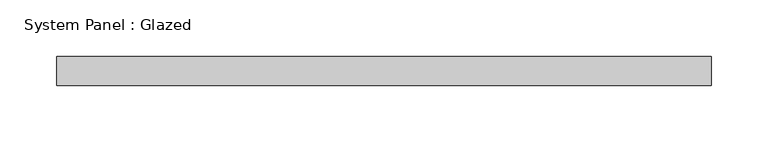
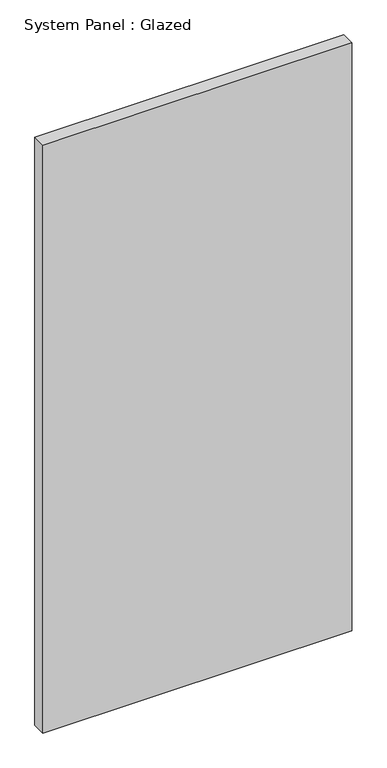
"""IFC4 building model written with IfcOpenShell, lengths in millimetres: plate geometry, System Panel : Glazed."""

from ifc_helpers import new_model, si_unit, origin, origin_with_axes, place, context, project, spatial, polyline, outline, extrude, source, transform, mapped, element, save


def system_panel_glazed_4d5e8b0b(model_context):
    return source(origin(), model_context, "Body", "SweptSolid", [
        extrude(outline(polyline([(287.1622579, 19.05), (-287.1622579, 19.05), (-287.1622579, 44.45), (287.1622579, 44.45), (287.1622579, 19.05)])), origin_with_axes(), (0.0, 0.0, 1.0), 1155.7),
    ])


if __name__ == "__main__":
    model = new_model("IFC4")
    model_context = context("Model", 3, world=origin())
    ifc_project = project(units=[si_unit("LENGTHUNIT", "METRE", prefix="MILLI")], contexts=[model_context])
    site = spatial("IfcSite", under=ifc_project)
    building = spatial("IfcBuilding", under=site)
    placement = place(None, origin())
    system_panel_glazed_shape = system_panel_glazed_4d5e8b0b(model_context)
    element("IfcPlate", 1, ObjectType="System Panel : Glazed", at=placement, inside=building, context=model_context, shape_type="MappedRepresentation", body=[
        mapped(system_panel_glazed_shape, transform((0.0, 0.0, 0.0), x_axis=(1.0, 0.0, 0.0), y_axis=(0.0, 1.0, 0.0), z_axis=(0.0, 0.0, 1.0))),
    ])
    save(model, "model.ifc")

# Revit data of these elements
# Type "System Panel : Glazed"
#   Construction Type Id = "GSP4R"
#   Analytic Construction = "1/8 in Pilkington single glazing"
#   Visual Light Transmittance = 0.9
#   Solar Heat Gain Coefficient = 0.86
#   Heat Transfer Coefficient (U) = 1.18115 BTU/(h·ft²·°F)
# Element 1 (IfcPlate, "System Panel : Glazed")
#   Materials on its faces: "Glass"
# Materials
#   "Glass": class "Glass", colour RGB 0 128 192, transparency 0.75, Description = "Soda Lime Glass", Cost = 0
